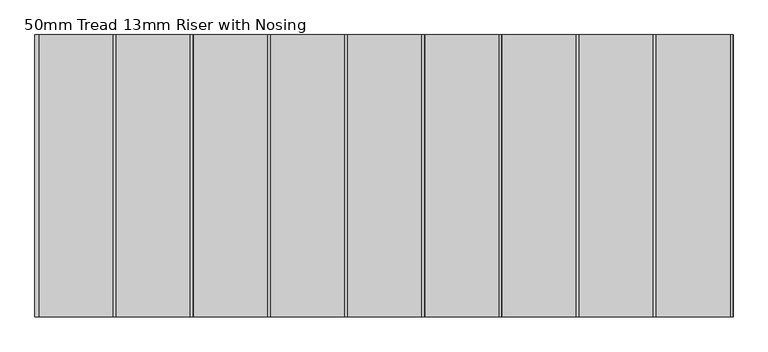
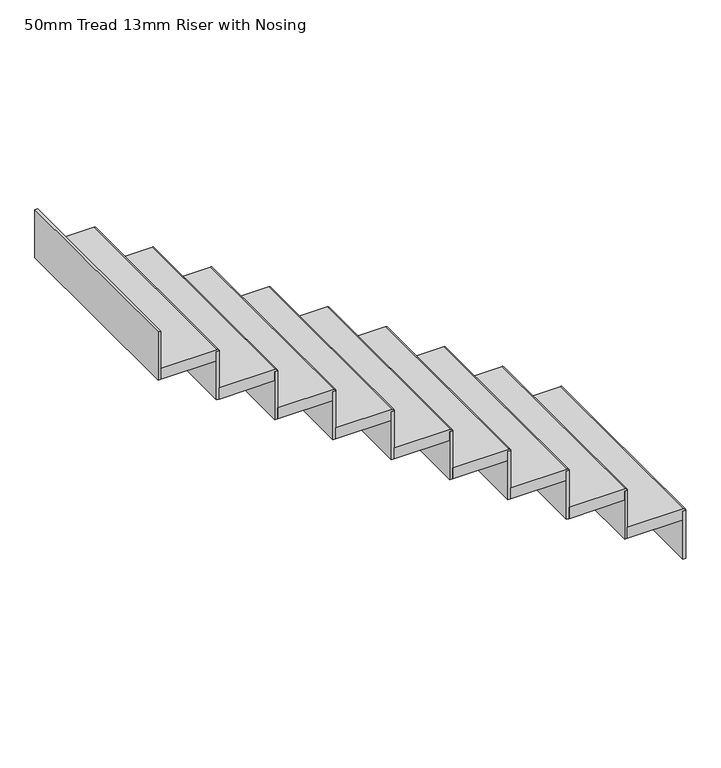
"""IFC4 building model written with IfcOpenShell, lengths in millimetres: stair flight geometry, 50mm Tread 13mm Riser with Nosing."""

from ifc_helpers import new_model, si_unit, point, frame, frame_2d, origin, place, context, project, spatial, polyline, circle_curve, trimmed, segment, composite_curve, outline, extrude, source, transform, mapped, element, save


def stair_flight_50mm_tread_13mm_riser_with_nosing_ea10009b(model_context):
    return source(origin(), model_context, "Body", "SweptSolid", [
        extrude(outline(polyline([(-7566.7282945, -3323.3921603), (-7554.2282945, -3323.3921603), (-7554.2282945, -4237.7921603), (-7566.7282945, -4237.7921603), (-7566.7282945, -3323.3921603)])), frame((0.0, 0.0, 1728.0), z_axis=(0.0, 0.0, 1.0), x_axis=(1.0, 0.0, 0.0)), (0.0, 0.0, 1.0), 217.8),
        extrude(outline(composite_curve([segment(polyline([(1955.8, -7564.2282945), (1955.8, -7804.2282945), (1905.8, -7804.2282945), (1905.8, -7564.2282945), (1935.8, -7564.2282945)]), True, "CONTINUOUS"), segment(trimmed(circle_curve(frame_2d((1945.8, -7564.2282945)), 10.0), [point((1935.8, -7564.2282945))], [point((1955.8, -7564.2282945))], False, "CARTESIAN"), True, "CONTINUOUS")], self_intersect=False)), frame((0.0, -4237.7921603, 0.0), z_axis=(0.0, 1.0, 0.0), x_axis=(0.0, 0.0, 1.0)), (0.0, 0.0, 1.0), 914.4),
        extrude(outline(polyline([(-7816.7282945, -3323.3921603), (-7804.2282945, -3323.3921603), (-7804.2282945, -4237.7921603), (-7816.7282945, -4237.7921603), (-7816.7282945, -3323.3921603)])), frame((0.0, 0.0, 1905.8), z_axis=(0.0, 0.0, 1.0), x_axis=(1.0, 0.0, 0.0)), (0.0, 0.0, 1.0), 217.8),
        extrude(outline(composite_curve([segment(polyline([(2133.6, -7814.2282945), (2133.6, -8054.2282945), (2083.6, -8054.2282945), (2083.6, -7814.2282945), (2113.6, -7814.2282945)]), True, "CONTINUOUS"), segment(trimmed(circle_curve(frame_2d((2123.6, -7814.2282945)), 10.0), [point((2113.6, -7814.2282945))], [point((2133.6, -7814.2282945))], False, "CARTESIAN"), True, "CONTINUOUS")], self_intersect=False)), frame((0.0, -4237.7921603, 0.0), z_axis=(0.0, 1.0, 0.0), x_axis=(0.0, 0.0, 1.0)), (0.0, 0.0, 1.0), 914.4),
        extrude(outline(polyline([(-8066.7282945, -3323.3921603), (-8054.2282945, -3323.3921603), (-8054.2282945, -4237.7921603), (-8066.7282945, -4237.7921603), (-8066.7282945, -3323.3921603)])), frame((0.0, 0.0, 2083.6), z_axis=(0.0, 0.0, 1.0), x_axis=(1.0, 0.0, 0.0)), (0.0, 0.0, 1.0), 217.8),
        extrude(outline(composite_curve([segment(polyline([(2311.4, -8064.2282945), (2311.4, -8304.2282945), (2261.4, -8304.2282945), (2261.4, -8064.2282945), (2291.4, -8064.2282945)]), True, "CONTINUOUS"), segment(trimmed(circle_curve(frame_2d((2301.4, -8064.2282945)), 10.0), [point((2291.4, -8064.2282945))], [point((2311.4, -8064.2282945))], False, "CARTESIAN"), True, "CONTINUOUS")], self_intersect=False)), frame((0.0, -4237.7921603, 0.0), z_axis=(0.0, 1.0, 0.0), x_axis=(0.0, 0.0, 1.0)), (0.0, 0.0, 1.0), 914.4),
        extrude(outline(polyline([(-8316.7282945, -3323.3921603), (-8304.2282945, -3323.3921603), (-8304.2282945, -4237.7921603), (-8316.7282945, -4237.7921603), (-8316.7282945, -3323.3921603)])), frame((0.0, 0.0, 2261.4), z_axis=(0.0, 0.0, 1.0), x_axis=(1.0, 0.0, 0.0)), (0.0, 0.0, 1.0), 217.8),
        extrude(outline(composite_curve([segment(polyline([(2489.2, -8314.2282945), (2489.2, -8554.2282945), (2439.2, -8554.2282945), (2439.2, -8314.2282945), (2469.2, -8314.2282945)]), True, "CONTINUOUS"), segment(trimmed(circle_curve(frame_2d((2479.2, -8314.2282945)), 10.0), [point((2469.2, -8314.2282945))], [point((2489.2, -8314.2282945))], False, "CARTESIAN"), True, "CONTINUOUS")], self_intersect=False)), frame((0.0, -4237.7921603, 0.0), z_axis=(0.0, 1.0, 0.0), x_axis=(0.0, 0.0, 1.0)), (0.0, 0.0, 1.0), 914.4),
        extrude(outline(polyline([(-8566.7282945, -3323.3921603), (-8554.2282945, -3323.3921603), (-8554.2282945, -4237.7921603), (-8566.7282945, -4237.7921603), (-8566.7282945, -3323.3921603)])), frame((0.0, 0.0, 2439.2), z_axis=(0.0, 0.0, 1.0), x_axis=(1.0, 0.0, 0.0)), (0.0, 0.0, 1.0), 217.8),
        extrude(outline(composite_curve([segment(polyline([(2667.0, -8564.2282945), (2667.0, -8804.2282945), (2617.0, -8804.2282945), (2617.0, -8564.2282945), (2647.0, -8564.2282945)]), True, "CONTINUOUS"), segment(trimmed(circle_curve(frame_2d((2657.0, -8564.2282945)), 10.0), [point((2647.0, -8564.2282945))], [point((2667.0, -8564.2282945))], False, "CARTESIAN"), True, "CONTINUOUS")], self_intersect=False)), frame((0.0, -4237.7921603, 0.0), z_axis=(0.0, 1.0, 0.0), x_axis=(0.0, 0.0, 1.0)), (0.0, 0.0, 1.0), 914.4),
        extrude(outline(polyline([(-8816.7282945, -3323.3921603), (-8804.2282945, -3323.3921603), (-8804.2282945, -4237.7921603), (-8816.7282945, -4237.7921603), (-8816.7282945, -3323.3921603)])), frame((0.0, 0.0, 2617.0), z_axis=(0.0, 0.0, 1.0), x_axis=(1.0, 0.0, 0.0)), (0.0, 0.0, 1.0), 217.8),
        extrude(outline(composite_curve([segment(polyline([(2844.8, -8814.2282945), (2844.8, -9054.2282945), (2794.8, -9054.2282945), (2794.8, -8814.2282945), (2824.8, -8814.2282945)]), True, "CONTINUOUS"), segment(trimmed(circle_curve(frame_2d((2834.8, -8814.2282945)), 10.0), [point((2824.8, -8814.2282945))], [point((2844.8, -8814.2282945))], False, "CARTESIAN"), True, "CONTINUOUS")], self_intersect=False)), frame((0.0, -4237.7921603, 0.0), z_axis=(0.0, 1.0, 0.0), x_axis=(0.0, 0.0, 1.0)), (0.0, 0.0, 1.0), 914.4),
        extrude(outline(polyline([(-9066.7282945, -3323.3921603), (-9054.2282945, -3323.3921603), (-9054.2282945, -4237.7921603), (-9066.7282945, -4237.7921603), (-9066.7282945, -3323.3921603)])), frame((0.0, 0.0, 2794.8), z_axis=(0.0, 0.0, 1.0), x_axis=(1.0, 0.0, 0.0)), (0.0, 0.0, 1.0), 217.8),
        extrude(outline(composite_curve([segment(polyline([(3022.6, -9064.2282945), (3022.6, -9304.2282945), (2972.6, -9304.2282945), (2972.6, -9064.2282945), (3002.6, -9064.2282945)]), True, "CONTINUOUS"), segment(trimmed(circle_curve(frame_2d((3012.6, -9064.2282945)), 10.0), [point((3002.6, -9064.2282945))], [point((3022.6, -9064.2282945))], False, "CARTESIAN"), True, "CONTINUOUS")], self_intersect=False)), frame((0.0, -4237.7921603, 0.0), z_axis=(0.0, 1.0, 0.0), x_axis=(0.0, 0.0, 1.0)), (0.0, 0.0, 1.0), 914.4),
        extrude(outline(polyline([(-9316.7282945, -3323.3921603), (-9304.2282945, -3323.3921603), (-9304.2282945, -4237.7921603), (-9316.7282945, -4237.7921603), (-9316.7282945, -3323.3921603)])), frame((0.0, 0.0, 2972.6), z_axis=(0.0, 0.0, 1.0), x_axis=(1.0, 0.0, 0.0)), (0.0, 0.0, 1.0), 217.8),
        extrude(outline(composite_curve([segment(polyline([(3200.4, -9314.2282945), (3200.4, -9554.2282945), (3150.4, -9554.2282945), (3150.4, -9314.2282945), (3180.4, -9314.2282945)]), True, "CONTINUOUS"), segment(trimmed(circle_curve(frame_2d((3190.4, -9314.2282945)), 10.0), [point((3180.4, -9314.2282945))], [point((3200.4, -9314.2282945))], False, "CARTESIAN"), True, "CONTINUOUS")], self_intersect=False)), frame((0.0, -4237.7921603, 0.0), z_axis=(0.0, 1.0, 0.0), x_axis=(0.0, 0.0, 1.0)), (0.0, 0.0, 1.0), 914.4),
        extrude(outline(polyline([(-9566.7282945, -3323.3921603), (-9554.2282945, -3323.3921603), (-9554.2282945, -4237.7921603), (-9566.7282945, -4237.7921603), (-9566.7282945, -3323.3921603)])), frame((0.0, 0.0, 3150.4), z_axis=(0.0, 0.0, 1.0), x_axis=(1.0, 0.0, 0.0)), (0.0, 0.0, 1.0), 217.8),
        extrude(outline(polyline([(-9816.7282945, -3323.3921603), (-9804.2282945, -3323.3921603), (-9804.2282945, -4237.7921603), (-9816.7282945, -4237.7921603), (-9816.7282945, -3323.3921603)])), frame((0.0, 0.0, 3328.2), z_axis=(0.0, 0.0, 1.0), x_axis=(1.0, 0.0, 0.0)), (0.0, 0.0, 1.0), 217.8),
        extrude(outline(composite_curve([segment(polyline([(3378.2, -9564.2282945), (3378.2, -9804.2282945), (3328.2, -9804.2282945), (3328.2, -9564.2282945), (3358.2, -9564.2282945)]), True, "CONTINUOUS"), segment(trimmed(circle_curve(frame_2d((3368.2, -9564.2282945)), 10.0), [point((3358.2, -9564.2282945))], [point((3378.2, -9564.2282945))], False, "CARTESIAN"), True, "CONTINUOUS")], self_intersect=False)), frame((0.0, -4237.7921603, 0.0), z_axis=(0.0, 1.0, 0.0), x_axis=(0.0, 0.0, 1.0)), (0.0, 0.0, 1.0), 914.4),
    ])


if __name__ == "__main__":
    model = new_model("IFC4")
    model_context = context("Model", 3, world=origin())
    ifc_project = project(units=[si_unit("LENGTHUNIT", "METRE", prefix="MILLI")], contexts=[model_context])
    site = spatial("IfcSite", under=ifc_project)
    building = spatial("IfcBuilding", under=site)
    placement = place(None, origin())
    stair_flight_50mm_tread_13mm_riser_with_nosing_shape = stair_flight_50mm_tread_13mm_riser_with_nosing_ea10009b(model_context)
    element("IfcStairFlight", 1, ObjectType="50mm Tread 13mm Riser with Nosing", at=placement, inside=building, context=model_context, shape_type="MappedRepresentation", body=[
        mapped(stair_flight_50mm_tread_13mm_riser_with_nosing_shape, transform((0.0, 0.0, 0.0), x_axis=(1.0, 0.0, 0.0), y_axis=(0.0, 1.0, 0.0), z_axis=(0.0, 0.0, 1.0))),
    ])
    save(model, "model.ifc")
